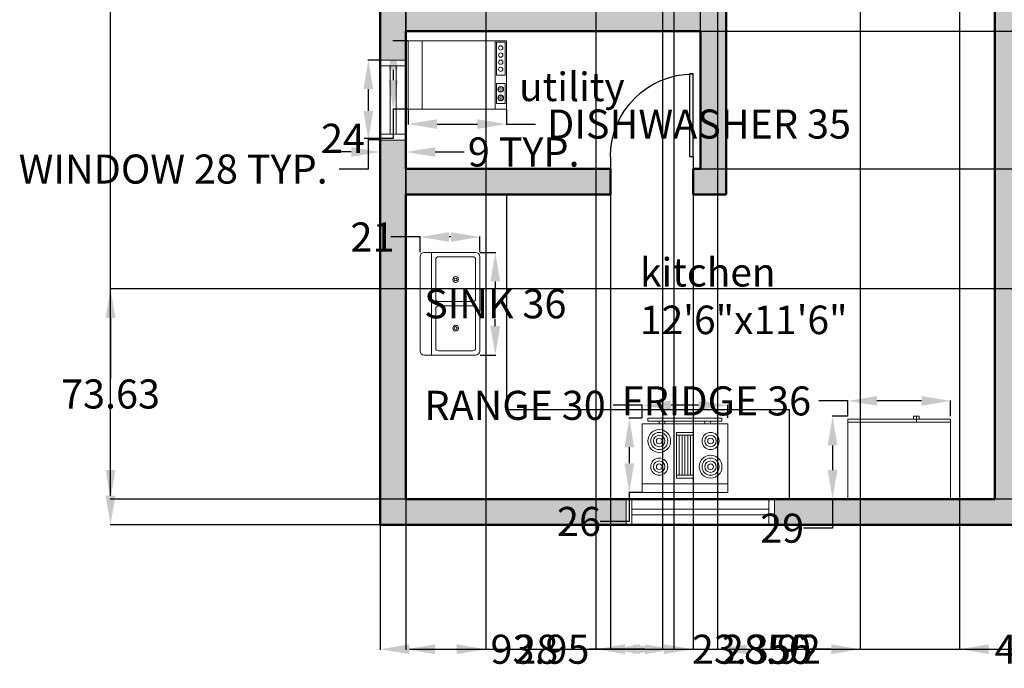
# Model space of a CAD drawing. Units: inches. Extents: x 12496 to 13538, y 6171 to 6892.
# Tile 1 of 6: x 12496 to 12841, y 6171 to 6398. Entities that reach past the tile are written whole.
import ezdxf

# ---------------------------------------------------------------- set-up
doc = ezdxf.new("R2010")
doc.units = ezdxf.units.IN
doc.header["$MEASUREMENT"] = 0
for name, color, linetype, lineweight in [('A-ANNO-DIMS', 2, 'Continuous', 18), ('A-AREA-IDEN', 7, 'Continuous', 25), ('A-DOOR', 3, 'Continuous', 25), ('A-EQPM', 8, 'Continuous', 18), ('A-FLOR-CASE', 8, 'Continuous', 25), ('A-FLOR-FIXT', 9, 'Continuous', 18), ('A-GLAZ', 4, 'Continuous', 18), ('A-WALL', 7, 'Continuous', 50)]:
    doc.layers.add(name, color=color, linetype=linetype, lineweight=lineweight)
doc.layers.add('A-WALL-PATT', color=18, linetype='Continuous', lineweight=13, true_color=0x000000)
doc.styles.get("Standard").update_dxf_attribs({"font": 'arial.ttf'})
doc.dimstyles.get("Standard").update_dxf_attribs({"dimtxt": 10.18, "dimasz": 10.18, "dimexe": 0.18, "dimexo": 0.0625, "dimgap": 0.09, "dimtad": 0, "dimtih": 1, "dimtoh": 1, "dimdec": 0, "dimzin": 0, "dimdsep": 46, "dimlunit": 3, "dimtxsty": 'Standard', "dimcen": 0.09, "dimadec": 0, "dimazin": 0, "dimtfac": 1, "dimtdec": 0, "dimtofl": 0, "dimtmove": 0, "dimatfit": 3, "dimfxl": 1, "dimtolj": 1, "dimtzin": 0, "dimarcsym": 0})

# ---------------------------------------------------------------- blocks, each defined once
blk = doc.blocks.new('Range-Oven - 30 in top')
for p, q in [((0, -3), (30, -3)), ((12, -6), (18, -6)), ((13, -20), (13, -6)), ((14, -6), (14, -20)), ((15, -20), (15, -6)), ((16, -6), (16, -20)), ((17, -20), (17, -6)), ((18, -20), (12, -20)), ((6, -24), (6, -25)), ((8, -25), (8, -24)), ((22, -25), (22, -24)), ((24, -24), (24, -25))]:
    blk.add_line(p, q)
for points in [[(0, -24), (0, 0), (30, 0), (30, -24)], [(12, -21), (12, -5), (18, -5), (18, -21)], [(2, -26), (2, -25), (28, -25), (28, -26)]]:
    blk.add_lwpolyline(points, close=True)
for centre, radius in [((6, -9), 4), ((6, -9), 3), ((24, -9), 3), ((6, -9), 2), ((6, -9), 1), ((24, -9), 2), ((24, -9), 1), ((6, -18), 3), ((6, -18), 2), ((6, -18), 1), ((24, -18), 4), ((24, -18), 3), ((24, -18), 2), ((24, -18), 1)]:
    blk.add_circle(centre, radius)
blk = doc.blocks.new('Sink-double - 36 in top')
for p, q in [((-18, -4), (18, -4)), ((-0.75, -18.5), (-0.75, -6.5)), ((0.75, -6.5), (0.75, -18.5))]:
    blk.add_line(p, q)
for points in [[(-16.5, 0), (16.5, 0)], [(-18, -19.5), (-18, -1.5)], [(18, -1.5), (18, -19.5)], [(-16.5, -18.5), (-16.5, -6.5)], [(-15.5, -5.5), (-1.75, -5.5)], [(1.75, -5.5), (15.5, -5.5)], [(16.5, -6.5), (16.5, -18.5)], [(-1.75, -19.5), (-15.5, -19.5)], [(15.5, -19.5), (1.75, -19.5)], [(16.5, -21), (-16.5, -21)]]:
    blk.add_lwpolyline(points)
for centre, radius in [((-8.5, -12.5), 1), ((-8.5, -12.5), 0.5), ((8.5, -12.5), 1), ((8.5, -12.5), 0.5)]:
    blk.add_circle(centre, radius)
for centre, radius, start, end in [((-16.5, -1.5), 1.5, 90, 180), ((16.5, -1.5), 1.5, 0, 90), ((-15.5, -6.5), 1, 90, 180), ((-1.75, -6.5), 1, 0, 90), ((1.75, -6.5), 1, 90, 180), ((15.5, -6.5), 1, 0, 90), ((-16.5, -19.5), 1.5, 180, 270), ((-15.5, -18.5), 1, 180, 270), ((-1.75, -18.5), 1, 270, 0), ((1.75, -18.5), 1, 180, 270), ((15.5, -18.5), 1, 270, 0), ((16.5, -19.5), 1.5, 270, 0)]:
    blk.add_arc(centre, radius, start, end)
blk = doc.blocks.new('Refrigerator-2 door - 36 in top')
for p, q in [((0, -26.999999), (36, -26.999999)), ((12, -26.999999), (12, -28.999999)), ((11, -27.999999), (11, -28.999999)), ((11, -28.999999), (13, -28.999999)), ((13, -28.999999), (13, -27.999999))]:
    blk.add_line(p, q)
blk.add_lwpolyline([(0, -27.999999), (0, 0), (36, 0), (36, -27.999999)], close=True)
blk = doc.blocks.new('Dishwasher')
for p, q in [((16, 32.5), (16.75, 32.5)), ((16.5, 32), (16.2942, 31.7942)), ((16.3156, 33.1843), (16.5, 33)), ((17, 32.75), (17, 33.5)), ((17, 32.25), (17, 31.5)), ((18, 32.5), (17.25, 32.5)), ((17.5, 33), (17.6938, 33.1938)), ((17.7061, 31.7939), (17.5, 32)), ((19, 32.5), (19.75, 32.5)), ((19.5, 32), (19.2942, 31.7942)), ((19.3156, 33.1843), (19.5, 33)), ((20, 32.75), (20, 33.5)), ((20, 32.25), (20, 31.5)), ((21, 32.5), (20.25, 32.5)), ((20.5, 33), (20.6938, 33.1938)), ((20.7061, 31.7939), (20.5, 32)), ((24, 30.5), (0, 30.5)), ((0, 5), (24, 5))]:
    blk.add_line(p, q)
for points in [[(0, 0), (0, 34.5), (24, 34.5), (24, 0)], [(0.5, 31), (0.5, 34), (12, 34), (12, 31)], [(15, 31), (15, 34), (22, 34), (22, 31)]]:
    blk.add_lwpolyline(points, close=True)
for centre, radius in [((2.5, 32.5), 0.75), ((5, 32.5), 0.75), ((7.5, 32.5), 0.75), ((10, 32.5), 0.75), ((17, 32.5), 1), ((20, 32.5), 1)]:
    blk.add_circle(centre, radius)
blk = doc.blocks.new('*U20')
for p, q in [((0, 0), (0, -6)), ((40, 0), (40, -6))]:
    blk.add_line(p, q)
blk.add_lwpolyline([(0, 0), (0, 40), (1.75, 40), (1.75, 0)], close=True)
blk.add_arc((0, 0), 40, 360, 90)
blk = doc.blocks.new('WIN-48IN')
for p, q in [((0, 0), (0, 9)), ((2, 0), (2, 9)), ((50, 0), (50, 9)), ((52, 0), (52, 9)), ((2, 5.5), (50, 5.5)), ((2, 3.5), (50, 3.5))]:
    blk.add_line(p, q)
blk = doc.blocks.new('WIN-24IN')
for p, q in [((0, 0), (0, 9)), ((2, 0), (2, 9)), ((26, 0), (26, 9)), ((28, 0), (28, 9)), ((2, 5.5), (26, 5.5)), ((2, 3.5), (26, 3.5))]:
    blk.add_line(p, q)
blk = doc.blocks.new('*D33')
at = {"layer": 'A-ANNO-DIMS', "color": 0, "lineweight": -2, "transparency": 16777216}
for p, q in [((12622.11, 6383.69), (12617.79, 6383.69)), ((12617.97, 6373.51), (12617.97, 6365.87)), ((12622.11, 6355.69), (12617.79, 6355.69)), ((12617.97, 6355.69), (12617.97, 6345.51)), ((12617.97, 6345.51), (12607.79, 6345.51))]:
    blk.add_line(p, q, dxfattribs=at)
at = {"layer": 'A-ANNO-DIMS', "color": 0, "transparency": 16777216}
for points in [[(12616.28, 6373.51), (12619.67, 6373.51), (12617.97, 6383.69)], [(12616.28, 6365.87), (12619.67, 6365.87), (12617.97, 6355.69)]]:
    blk.add_solid(points, dxfattribs=at)
at = {"layer": 'Defpoints', "color": 0, "transparency": 16777216}
for p in [(12622.17, 6383.69), (12617.97, 6355.69), (12622.17, 6355.69)]:
    blk.add_point(p, dxfattribs=at)
at = {"layer": 'A-ANNO-DIMS', "color": 0, "transparency": 16777216, "insert": (12549.54, 6345.51), "char_height": 10.18, "attachment_point": 5}
blk.add_mtext('\\A1;WINDOW 28 TYP.', dxfattribs=at)
blk = doc.blocks.new('*D34')
at = {"layer": 'A-ANNO-DIMS', "color": 0, "lineweight": -2, "transparency": 16777216}
for p, q in [((12622.17, 6355.62), (12622.17, 6351.31)), ((12631.17, 6355.62), (12631.17, 6351.31)), ((12611.99, 6351.49), (12601.81, 6351.49)), ((12641.35, 6351.49), (12651.53, 6351.49))]:
    blk.add_line(p, q, dxfattribs=at)
at = {"layer": 'A-ANNO-DIMS', "color": 0, "transparency": 16777216}
for points in [[(12611.99, 6353.18), (12611.99, 6349.79), (12622.17, 6351.49)], [(12641.35, 6353.18), (12641.35, 6349.79), (12631.17, 6351.49)]]:
    blk.add_solid(points, dxfattribs=at)
at = {"layer": 'Defpoints', "color": 0, "transparency": 16777216}
for p in [(12622.17, 6355.69), (12631.17, 6355.69), (12631.17, 6351.49)]:
    blk.add_point(p, dxfattribs=at)
at = {"layer": 'A-ANNO-DIMS', "color": 0, "transparency": 16777216, "insert": (12672.44, 6351.49), "char_height": 10.18, "attachment_point": 5}
blk.add_mtext('\\A1;9 TYP.', dxfattribs=at)
blk = doc.blocks.new('*D45')
at = {"layer": 'A-ANNO-DIMS', "color": 0, "lineweight": -2, "transparency": 16777216}
for p, q in [((12713.97, 6262.74), (12703.79, 6262.74)), ((12713.97, 6258.31), (12713.97, 6262.92)), ((12733.79, 6262.74), (12724.15, 6262.74)), ((12743.97, 6258.31), (12743.97, 6262.92))]:
    blk.add_line(p, q, dxfattribs=at)
at = {"layer": 'A-ANNO-DIMS', "color": 0, "transparency": 16777216}
for points in [[(12724.15, 6264.44), (12724.15, 6261.05), (12713.97, 6262.74)], [(12733.79, 6264.44), (12733.79, 6261.05), (12743.97, 6262.74)]]:
    blk.add_solid(points, dxfattribs=at)
at = {"layer": 'Defpoints', "color": 0, "transparency": 16777216}
for p in [(12713.97, 6262.74), (12713.97, 6258.24), (12743.97, 6258.24)]:
    blk.add_point(p, dxfattribs=at)
at = {"layer": 'A-ANNO-DIMS', "color": 0, "transparency": 16777216, "insert": (12669.43, 6262.74), "char_height": 10.18, "attachment_point": 5}
blk.add_mtext('\\A1;RANGE 30', dxfattribs=at)
blk = doc.blocks.new('*D46')
at = {"layer": 'A-ANNO-DIMS', "color": 0, "lineweight": -2, "transparency": 16777216}
for p, q in [((12713.91, 6258.24), (12709.29, 6258.24)), ((12709.47, 6248.06), (12709.47, 6242.42)), ((12713.91, 6232.24), (12709.29, 6232.24)), ((12709.47, 6232.24), (12709.47, 6222.06)), ((12709.47, 6222.06), (12699.29, 6222.06))]:
    blk.add_line(p, q, dxfattribs=at)
at = {"layer": 'A-ANNO-DIMS', "color": 0, "transparency": 16777216}
for points in [[(12707.77, 6248.06), (12711.17, 6248.06), (12709.47, 6258.24)], [(12707.77, 6242.42), (12711.17, 6242.42), (12709.47, 6232.24)]]:
    blk.add_solid(points, dxfattribs=at)
at = {"layer": 'Defpoints', "color": 0, "transparency": 16777216}
for p in [(12713.97, 6258.24), (12709.47, 6232.24), (12713.97, 6232.24)]:
    blk.add_point(p, dxfattribs=at)
at = {"layer": 'A-ANNO-DIMS', "color": 0, "transparency": 16777216, "insert": (12691.83, 6222.06), "char_height": 10.18, "attachment_point": 5}
blk.add_mtext('\\A1;26', dxfattribs=at)
blk = doc.blocks.new('*D47')
at = {"layer": 'A-ANNO-DIMS', "color": 0, "lineweight": -2, "transparency": 16777216}
for p, q in [((12657.15, 6316.31), (12662.67, 6316.31)), ((12662.49, 6306.13), (12662.49, 6303.67)), ((12662.49, 6290.49), (12662.49, 6292.96)), ((12657.15, 6280.31), (12662.67, 6280.31))]:
    blk.add_line(p, q, dxfattribs=at)
at = {"layer": 'A-ANNO-DIMS', "color": 0, "transparency": 16777216}
for points in [[(12660.79, 6306.13), (12664.19, 6306.13), (12662.49, 6316.31)], [(12660.79, 6290.49), (12664.19, 6290.49), (12662.49, 6280.31)]]:
    blk.add_solid(points, dxfattribs=at)
at = {"layer": 'Defpoints', "color": 0, "transparency": 16777216}
for p in [(12657.09, 6316.31), (12662.49, 6316.31), (12657.09, 6280.31)]:
    blk.add_point(p, dxfattribs=at)
at = {"layer": 'A-ANNO-DIMS', "color": 0, "transparency": 16777216, "insert": (12662.49, 6298.31), "char_height": 10.18, "attachment_point": 5}
blk.add_mtext('\\A1;SINK 36', dxfattribs=at)
blk = doc.blocks.new('*D48')
at = {"layer": 'A-ANNO-DIMS', "color": 0, "lineweight": -2, "transparency": 16777216}
for p, q in [((12636.09, 6321.71), (12625.91, 6321.71)), ((12636.09, 6316.38), (12636.09, 6321.89)), ((12646.91, 6321.71), (12646.27, 6321.71)), ((12657.09, 6316.38), (12657.09, 6321.89))]:
    blk.add_line(p, q, dxfattribs=at)
at = {"layer": 'A-ANNO-DIMS', "color": 0, "transparency": 16777216}
for points in [[(12646.27, 6323.41), (12646.27, 6320.02), (12636.09, 6321.71)], [(12646.91, 6323.41), (12646.91, 6320.02), (12657.09, 6321.71)]]:
    blk.add_solid(points, dxfattribs=at)
at = {"layer": 'Defpoints', "color": 0, "transparency": 16777216}
for p in [(12636.09, 6321.71), (12636.09, 6316.31), (12657.09, 6316.31)]:
    blk.add_point(p, dxfattribs=at)
at = {"layer": 'A-ANNO-DIMS', "color": 0, "transparency": 16777216, "insert": (12619.42, 6321.71), "char_height": 10.18, "attachment_point": 5}
blk.add_mtext('\\A1;21', dxfattribs=at)
blk = doc.blocks.new('*D49')
at = {"layer": 'A-ANNO-DIMS', "color": 0, "lineweight": -2, "transparency": 16777216}
for p, q in [((12786.13, 6264.29), (12775.95, 6264.29)), ((12786.13, 6258.96), (12786.13, 6264.47)), ((12811.95, 6264.29), (12796.31, 6264.29)), ((12822.13, 6258.96), (12822.13, 6264.47))]:
    blk.add_line(p, q, dxfattribs=at)
at = {"layer": 'A-ANNO-DIMS', "color": 0, "transparency": 16777216}
for points in [[(12796.31, 6265.99), (12796.31, 6262.6), (12786.13, 6264.29)], [(12811.95, 6265.99), (12811.95, 6262.6), (12822.13, 6264.29)]]:
    blk.add_solid(points, dxfattribs=at)
at = {"layer": 'Defpoints', "color": 0, "transparency": 16777216}
for p in [(12786.13, 6264.29), (12786.13, 6258.89), (12822.13, 6258.89)]:
    blk.add_point(p, dxfattribs=at)
at = {"layer": 'A-ANNO-DIMS', "color": 0, "transparency": 16777216, "insert": (12740.02, 6264.29), "char_height": 10.18, "attachment_point": 5}
blk.add_mtext('\\A1;FRIDGE 36', dxfattribs=at)
blk = doc.blocks.new('*D50')
at = {"layer": 'A-ANNO-DIMS', "color": 0, "lineweight": -2, "transparency": 16777216}
for p, q in [((12786.07, 6258.89), (12780.55, 6258.89)), ((12780.73, 6248.71), (12780.73, 6240.07)), ((12786.07, 6229.89), (12780.55, 6229.89)), ((12780.73, 6229.89), (12780.73, 6219.71)), ((12780.73, 6219.71), (12770.55, 6219.71))]:
    blk.add_line(p, q, dxfattribs=at)
at = {"layer": 'A-ANNO-DIMS', "color": 0, "transparency": 16777216}
for points in [[(12779.03, 6248.71), (12782.43, 6248.71), (12780.73, 6258.89)], [(12779.03, 6240.07), (12782.43, 6240.07), (12780.73, 6229.89)]]:
    blk.add_solid(points, dxfattribs=at)
at = {"layer": 'Defpoints', "color": 0, "transparency": 16777216}
for p in [(12786.13, 6258.89), (12780.73, 6229.89), (12786.13, 6229.89)]:
    blk.add_point(p, dxfattribs=at)
at = {"layer": 'A-ANNO-DIMS', "color": 0, "transparency": 16777216, "insert": (12763.07, 6219.71), "char_height": 10.18, "attachment_point": 5}
blk.add_mtext('\\A1;29', dxfattribs=at)
blk = doc.blocks.new('*D57')
at = {"layer": 'A-ANNO-DIMS', "color": 0, "lineweight": -2, "transparency": 16777216}
for p, q in [((12631.9, 6366.38), (12631.9, 6361.09)), ((12666.4, 6366.38), (12666.4, 6361.09)), ((12642.08, 6361.27), (12656.22, 6361.27)), ((12666.4, 6361.27), (12676.58, 6361.27))]:
    blk.add_line(p, q, dxfattribs=at)
at = {"layer": 'A-ANNO-DIMS', "color": 0, "transparency": 16777216}
for points in [[(12642.08, 6362.97), (12642.08, 6359.57), (12631.9, 6361.27)], [(12656.22, 6362.97), (12656.22, 6359.57), (12666.4, 6361.27)]]:
    blk.add_solid(points, dxfattribs=at)
at = {"layer": 'Defpoints', "color": 0, "transparency": 16777216}
for p in [(12631.9, 6366.45), (12666.4, 6366.45), (12666.4, 6361.27)]:
    blk.add_point(p, dxfattribs=at)
at = {"layer": 'A-ANNO-DIMS', "color": 0, "transparency": 16777216, "insert": (12733.92, 6361.27), "char_height": 10.18, "attachment_point": 5}
blk.add_mtext('\\A1;DISHWASHER 35', dxfattribs=at)
blk = doc.blocks.new('*D58')
at = {"layer": 'A-ANNO-DIMS', "color": 0, "lineweight": -2, "transparency": 16777216}
for p, q in [((12631.84, 6390.45), (12626.55, 6390.45)), ((12626.73, 6380.27), (12626.73, 6376.63)), ((12631.84, 6366.45), (12626.55, 6366.45)), ((12626.73, 6366.45), (12626.73, 6356.27)), ((12626.73, 6356.27), (12616.55, 6356.27))]:
    blk.add_line(p, q, dxfattribs=at)
at = {"layer": 'A-ANNO-DIMS', "color": 0, "transparency": 16777216}
for points in [[(12625.03, 6380.27), (12628.42, 6380.27), (12626.73, 6390.45)], [(12625.03, 6376.63), (12628.42, 6376.63), (12626.73, 6366.45)]]:
    blk.add_solid(points, dxfattribs=at)
at = {"layer": 'Defpoints', "color": 0, "transparency": 16777216}
for p in [(12631.9, 6390.45), (12626.73, 6366.45), (12631.9, 6366.45)]:
    blk.add_point(p, dxfattribs=at)
at = {"layer": 'A-ANNO-DIMS', "color": 0, "transparency": 16777216, "insert": (12609.1, 6356.27), "char_height": 10.18, "attachment_point": 5}
blk.add_mtext('\\A1;24', dxfattribs=at)
blk = doc.blocks.new('*D59')
at = {"layer": 'A-ANNO-DIMS', "color": 0, "lineweight": -2, "transparency": 16777216}
for p, q in [((12622.17, 6220.83), (12622.17, 6177.12)), ((13443.03, 6220.83), (13443.03, 6177.12)), ((12632.35, 6177.3), (13015.32, 6177.3)), ((13432.85, 6177.3), (13049.88, 6177.3))]:
    blk.add_line(p, q, dxfattribs=at)
at = {"layer": 'A-ANNO-DIMS', "color": 0, "transparency": 16777216}
for points in [[(12632.35, 6179), (12632.35, 6175.6), (12622.17, 6177.3)], [(13432.85, 6179), (13432.85, 6175.6), (13443.03, 6177.3)]]:
    blk.add_solid(points, dxfattribs=at)
at = {"layer": 'Defpoints', "color": 0, "transparency": 16777216}
for p in [(12622.17, 6220.89), (13443.03, 6220.89), (13443.03, 6177.3)]:
    blk.add_point(p, dxfattribs=at)
at = {"layer": 'A-ANNO-DIMS', "color": 0, "transparency": 16777216, "insert": (13032.6, 6177.3), "char_height": 10.18, "attachment_point": 5}
blk.add_mtext('\\A1;820.9', dxfattribs=at)
blk = doc.blocks.new('*D60')
at = {"layer": 'A-ANNO-DIMS', "color": 0, "lineweight": -2, "transparency": 16777216}
for p, q in [((12622.11, 6790.89), (12527.4, 6790.89)), ((12527.58, 6780.71), (12527.58, 6511.18)), ((12527.58, 6231.07), (12527.58, 6500.61)), ((12622.11, 6220.89), (12527.4, 6220.89))]:
    blk.add_line(p, q, dxfattribs=at)
at = {"layer": 'A-ANNO-DIMS', "color": 0, "transparency": 16777216}
for points in [[(12525.88, 6780.71), (12529.28, 6780.71), (12527.58, 6790.89)], [(12525.88, 6231.07), (12529.28, 6231.07), (12527.58, 6220.89)]]:
    blk.add_solid(points, dxfattribs=at)
at = {"layer": 'Defpoints', "color": 0, "transparency": 16777216}
for p in [(12527.58, 6790.89), (12622.17, 6790.89), (12622.17, 6220.89)]:
    blk.add_point(p, dxfattribs=at)
at = {"layer": 'A-ANNO-DIMS', "color": 0, "transparency": 16777216, "insert": (12527.58, 6505.89), "char_height": 10.18, "attachment_point": 5}
blk.add_mtext('\\A1;570', dxfattribs=at)
blk = doc.blocks.new('*D65')
at = {"layer": 'A-ANNO-DIMS', "color": 0, "lineweight": -2, "transparency": 16777216}
for p, q in [((12631.17, 6229.96), (12631.17, 6885.67)), ((12641.35, 6885.49), (12713.08, 6885.49)), ((12827.42, 6885.49), (12755.7, 6885.49)), ((12837.6, 6229.96), (12837.6, 6885.67))]:
    blk.add_line(p, q, dxfattribs=at)
at = {"layer": 'A-ANNO-DIMS', "color": 0, "transparency": 16777216}
for points in [[(12641.35, 6887.18), (12641.35, 6883.79), (12631.17, 6885.49)], [(12827.42, 6887.18), (12827.42, 6883.79), (12837.6, 6885.49)]]:
    blk.add_solid(points, dxfattribs=at)
at = {"layer": 'Defpoints', "color": 0, "transparency": 16777216}
for p in [(12837.6, 6885.49), (12631.17, 6229.89), (12837.6, 6229.89)]:
    blk.add_point(p, dxfattribs=at)
at = {"layer": 'A-ANNO-DIMS', "color": 0, "transparency": 16777216, "insert": (12734.39, 6885.49), "char_height": 10.18, "attachment_point": 5}
blk.add_mtext('\\A1;206.43', dxfattribs=at)
blk = doc.blocks.new('*D71')
at = {"layer": 'A-ANNO-DIMS', "color": 0, "lineweight": -2, "transparency": 16777216}
for p, q in [((13109.04, 6303.52), (12527.4, 6303.52)), ((12527.58, 6293.34), (12527.58, 6272)), ((12527.58, 6240.07), (12527.58, 6261.42)), ((13109.04, 6229.89), (12527.4, 6229.89))]:
    blk.add_line(p, q, dxfattribs=at)
at = {"layer": 'A-ANNO-DIMS', "color": 0, "transparency": 16777216}
for points in [[(12525.88, 6293.34), (12529.28, 6293.34), (12527.58, 6303.52)], [(12525.88, 6240.07), (12529.28, 6240.07), (12527.58, 6229.89)]]:
    blk.add_solid(points, dxfattribs=at)
at = {"layer": 'Defpoints', "color": 0, "transparency": 16777216}
for p in [(12527.58, 6303.52), (13109.1, 6303.52), (13109.1, 6229.89)]:
    blk.add_point(p, dxfattribs=at)
at = {"layer": 'A-ANNO-DIMS', "color": 0, "transparency": 16777216, "insert": (12527.58, 6266.71), "char_height": 10.18, "attachment_point": 5}
blk.add_mtext('\\A1;73.63', dxfattribs=at)
blk = doc.blocks.new('*D72')
at = {"layer": 'A-ANNO-DIMS', "color": 0, "lineweight": -2, "transparency": 16777216}
for p, q in [((12734.45, 6393.81), (13486.8, 6393.81)), ((13486.62, 6383.63), (13486.62, 6374.97)), ((13486.62, 6355.74), (13486.62, 6364.4)), ((12734.45, 6345.56), (13486.8, 6345.56))]:
    blk.add_line(p, q, dxfattribs=at)
at = {"layer": 'A-ANNO-DIMS', "color": 0, "transparency": 16777216}
for points in [[(13484.92, 6383.63), (13488.32, 6383.63), (13486.62, 6393.81)], [(13484.92, 6355.74), (13488.32, 6355.74), (13486.62, 6345.56)]]:
    blk.add_solid(points, dxfattribs=at)
at = {"layer": 'Defpoints', "color": 0, "transparency": 16777216}
for p in [(12734.39, 6393.81), (13486.62, 6393.81), (12734.39, 6345.56)]:
    blk.add_point(p, dxfattribs=at)
at = {"layer": 'A-ANNO-DIMS', "color": 0, "transparency": 16777216, "insert": (13486.62, 6369.69), "char_height": 10.18, "attachment_point": 5}
blk.add_mtext('\\A1;48.25', dxfattribs=at)
blk = doc.blocks.new('*D73')
at = {"layer": 'A-ANNO-DIMS', "color": 0, "lineweight": -2, "transparency": 16777216}
for p, q in [((12631.17, 6393.87), (12631.17, 6885.67)), ((12641.35, 6885.49), (12663.02, 6885.49)), ((12724.21, 6885.49), (12702.54, 6885.49)), ((12734.39, 6393.87), (12734.39, 6885.67))]:
    blk.add_line(p, q, dxfattribs=at)
at = {"layer": 'A-ANNO-DIMS', "color": 0, "transparency": 16777216}
for points in [[(12641.35, 6887.18), (12641.35, 6883.79), (12631.17, 6885.49)], [(12724.21, 6887.18), (12724.21, 6883.79), (12734.39, 6885.49)]]:
    blk.add_solid(points, dxfattribs=at)
at = {"layer": 'Defpoints', "color": 0, "transparency": 16777216}
for p in [(12734.39, 6885.49), (12631.17, 6393.81), (12734.39, 6393.81)]:
    blk.add_point(p, dxfattribs=at)
at = {"layer": 'A-ANNO-DIMS', "color": 0, "transparency": 16777216, "insert": (12682.78, 6885.49), "char_height": 10.18, "attachment_point": 5}
blk.add_mtext('\\A1;103.21', dxfattribs=at)
blk = doc.blocks.new('*D74')
at = {"layer": 'A-ANNO-DIMS', "color": 0, "lineweight": -2, "transparency": 16777216}
for p, q in [((12702.9, 6345.5), (12702.9, 6177.12)), ((12731.82, 6345.5), (12731.82, 6177.12)), ((12713.08, 6177.3), (12721.64, 6177.3)), ((12731.82, 6177.3), (12742, 6177.3))]:
    blk.add_line(p, q, dxfattribs=at)
at = {"layer": 'A-ANNO-DIMS', "color": 0, "transparency": 16777216}
for points in [[(12713.08, 6179), (12713.08, 6175.6), (12702.9, 6177.3)], [(12721.64, 6179), (12721.64, 6175.6), (12731.82, 6177.3)]]:
    blk.add_solid(points, dxfattribs=at)
at = {"layer": 'Defpoints', "color": 0, "transparency": 16777216}
for p in [(12702.9, 6345.56), (12731.82, 6345.56), (12731.82, 6177.3)]:
    blk.add_point(p, dxfattribs=at)
at = {"layer": 'A-ANNO-DIMS', "color": 0, "transparency": 16777216, "insert": (12759.3, 6177.3), "char_height": 10.18, "attachment_point": 5}
blk.add_mtext('\\A1;28.92', dxfattribs=at)
blk = doc.blocks.new('*D77')
at = {"layer": 'A-ANNO-DIMS', "color": 0, "lineweight": -2, "transparency": 16777216}
for p, q in [((12697.73, 6559.71), (12697.73, 6177.12)), ((12721.09, 6560.6), (12721.09, 6177.12)), ((12707.91, 6177.3), (12710.91, 6177.3)), ((12721.09, 6177.3), (12731.27, 6177.3))]:
    blk.add_line(p, q, dxfattribs=at)
at = {"layer": 'A-ANNO-DIMS', "color": 0, "transparency": 16777216}
for points in [[(12707.91, 6179), (12707.91, 6175.6), (12697.73, 6177.3)], [(12710.91, 6179), (12710.91, 6175.6), (12721.09, 6177.3)]]:
    blk.add_solid(points, dxfattribs=at)
at = {"layer": 'Defpoints', "color": 0, "transparency": 16777216}
for p in [(12697.73, 6559.77), (12721.09, 6560.66), (12721.09, 6177.3)]:
    blk.add_point(p, dxfattribs=at)
at = {"layer": 'A-ANNO-DIMS', "color": 0, "transparency": 16777216, "insert": (12752.61, 6177.3), "char_height": 10.18, "attachment_point": 5}
blk.add_mtext('\\A1;23.355', dxfattribs=at)
blk = doc.blocks.new('*D79')
at = {"layer": 'A-ANNO-DIMS', "color": 0, "lineweight": -2, "transparency": 16777216}
for p, q in [((12659.17, 6539.09), (12659.17, 6177.12)), ((12631.17, 6528.59), (12631.17, 6177.12)), ((12641.35, 6177.3), (12648.99, 6177.3)), ((12659.17, 6177.3), (12669.35, 6177.3))]:
    blk.add_line(p, q, dxfattribs=at)
at = {"layer": 'A-ANNO-DIMS', "color": 0, "transparency": 16777216}
for points in [[(12641.35, 6179), (12641.35, 6175.6), (12631.17, 6177.3)], [(12648.99, 6179), (12648.99, 6175.6), (12659.17, 6177.3)]]:
    blk.add_solid(points, dxfattribs=at)
at = {"layer": 'Defpoints', "color": 0, "transparency": 16777216}
for p in [(12659.17, 6539.15), (12631.17, 6528.65), (12659.17, 6177.3)]:
    blk.add_point(p, dxfattribs=at)
at = {"layer": 'A-ANNO-DIMS', "color": 0, "transparency": 16777216, "insert": (12676.83, 6177.3), "char_height": 10.18, "attachment_point": 5}
blk.add_mtext('\\A1;28', dxfattribs=at)
blk = doc.blocks.new('*D80')
at = {"layer": 'A-ANNO-DIMS', "color": 0, "lineweight": -2, "transparency": 16777216}
for p, q in [((12631.17, 6781.83), (12631.17, 6177.12)), ((12725.12, 6781.83), (12725.12, 6177.12)), ((12641.35, 6177.3), (12660.84, 6177.3)), ((12714.94, 6177.3), (12695.45, 6177.3))]:
    blk.add_line(p, q, dxfattribs=at)
at = {"layer": 'A-ANNO-DIMS', "color": 0, "transparency": 16777216}
for points in [[(12641.35, 6179), (12641.35, 6175.6), (12631.17, 6177.3)], [(12714.94, 6179), (12714.94, 6175.6), (12725.12, 6177.3)]]:
    blk.add_solid(points, dxfattribs=at)
at = {"layer": 'Defpoints', "color": 0, "transparency": 16777216}
for p in [(12631.17, 6781.89), (12725.12, 6781.89), (12725.12, 6177.3)]:
    blk.add_point(p, dxfattribs=at)
at = {"layer": 'A-ANNO-DIMS', "color": 0, "transparency": 16777216, "insert": (12678.15, 6177.3), "char_height": 10.18, "attachment_point": 5}
blk.add_mtext('\\A1;93.95', dxfattribs=at)
blk = doc.blocks.new('*D86')
at = {"layer": 'A-ANNO-DIMS', "color": 0, "lineweight": -2, "transparency": 16777216}
for p, q in [((12740.45, 6507.47), (12740.45, 6177.12)), ((12790.45, 6507.47), (12790.45, 6177.12)), ((12750.63, 6177.3), (12758.09, 6177.3)), ((12780.27, 6177.3), (12772.81, 6177.3))]:
    blk.add_line(p, q, dxfattribs=at)
at = {"layer": 'A-ANNO-DIMS', "color": 0, "transparency": 16777216}
for points in [[(12750.63, 6179), (12750.63, 6175.6), (12740.45, 6177.3)], [(12780.27, 6179), (12780.27, 6175.6), (12790.45, 6177.3)]]:
    blk.add_solid(points, dxfattribs=at)
at = {"layer": 'Defpoints', "color": 0, "transparency": 16777216}
for p in [(12740.45, 6507.54), (12790.45, 6507.54), (12790.45, 6177.3)]:
    blk.add_point(p, dxfattribs=at)
at = {"layer": 'A-ANNO-DIMS', "color": 0, "transparency": 16777216, "insert": (12765.45, 6177.3), "char_height": 10.18, "attachment_point": 5}
blk.add_mtext('\\A1;50', dxfattribs=at)
blk = doc.blocks.new('*D87')
at = {"layer": 'A-ANNO-DIMS', "color": 0, "lineweight": -2, "transparency": 16777216}
for p, q in [((12825.27, 6572.14), (12825.27, 6177.12)), ((12865.27, 6572.14), (12865.27, 6177.12)), ((12835.45, 6177.3), (12837.7, 6177.3)), ((12855.09, 6177.3), (12852.83, 6177.3))]:
    blk.add_line(p, q, dxfattribs=at)
at = {"layer": 'A-ANNO-DIMS', "color": 0, "transparency": 16777216}
for points in [[(12835.45, 6179), (12835.45, 6175.6), (12825.27, 6177.3)], [(12855.09, 6179), (12855.09, 6175.6), (12865.27, 6177.3)]]:
    blk.add_solid(points, dxfattribs=at)
at = {"layer": 'Defpoints', "color": 0, "transparency": 16777216}
for p in [(12825.27, 6572.2), (12865.27, 6572.2), (12865.27, 6177.3)]:
    blk.add_point(p, dxfattribs=at)
at = {"layer": 'A-ANNO-DIMS', "color": 0, "transparency": 16777216, "insert": (12845.27, 6177.3), "char_height": 10.18, "attachment_point": 5}
blk.add_mtext('\\A1;40', dxfattribs=at)

msp = doc.modelspace()

# ---------------------------------------------------------------- hatches: boundary and pattern name
at = {"layer": 'A-WALL-PATT'}
h = msp.add_hatch(color=256, dxfattribs=at)
h.dxf.hatch_style = 1
h.paths.add_polyline_path([(13443.0285, 6790.8943), (13327.7025, 6790.8943), (13327.7025, 6781.8943), (13434.0285, 6781.8943), (13434.0285, 6572.2028), (13169.3765, 6572.2028), (13169.3765, 6576.9323), (13160.3765, 6576.9323), (13160.3765, 6563.2028), (13163.811, 6563.2028), (13163.811, 6559.305), (13172.811, 6559.305), (13172.811, 6563.2028), (13434.0285, 6563.2028), (13434.0285, 6402.794), (13331.4198, 6402.794), (13331.4198, 6393.8103), (13434.0285, 6393.8103), (13434.0285, 6220.8943), (13443.0285, 6220.8943)])
h.paths.add_polyline_path([(13172.811, 6519.305), (13163.811, 6519.305), (13163.811, 6402.8103), (12944.6655, 6402.8103), (12944.6655, 6393.8103), (13100.0985, 6393.8103), (13100.0985, 6312.5223), (13035.7682, 6312.5223), (13035.7682, 6303.5223), (13109.0985, 6303.5223), (13109.0985, 6393.8103), (13279.4198, 6393.8103), (13279.4198, 6402.8103), (13172.811, 6402.8103)])
h.paths.add_polyline_path([(13109.0985, 6229.8943), (12846.603, 6229.8943), (12846.603, 6303.5223), (12853.6371, 6303.5223), (12853.6371, 6312.5223), (12846.603, 6312.5223), (12846.603, 6393.8103), (12872.7237, 6393.8103), (12872.7237, 6402.8103), (12846.603, 6402.8103), (12837.603, 6402.8103), (12837.603, 6229.8943), (12760.3881, 6229.8943), (12760.3881, 6220.8943), (13109.0985, 6220.8943)])
h.paths.add_polyline_path([(12708.3881, 6229.8943), (12631.1731, 6229.8943), (12631.1731, 6336.5598), (12702.8967, 6336.5598), (12702.8967, 6345.5598), (12631.1731, 6345.5598), (12631.1731, 6355.6851), (12622.1731, 6355.6851), (12622.1731, 6220.8943), (12708.3881, 6220.8943)])
h.paths.add_polyline_path([(12743.3881, 6402.8103), (12631.1731, 6402.8103), (12631.1731, 6523.6486), (12622.1731, 6523.6486), (12622.1731, 6383.6851), (12631.1731, 6383.6851), (12631.1731, 6393.8103), (12734.3881, 6393.8103), (12734.3881, 6345.5598), (12731.8151, 6345.5598), (12731.8151, 6336.5598), (12734.3881, 6336.5598), (12743.3881, 6336.5598)])
h.paths.add_polyline_path([(13039.9206, 6572.2028), (13039.9206, 6638.8628), (13048.7069, 6638.8628), (13048.7069, 6647.8628), (13039.9206, 6647.8628), (12930.9211, 6647.8628), (12930.9211, 6638.8628), (13030.9206, 6638.8628), (13030.9206, 6572.2028), (12880.0706, 6572.2028), (12880.0706, 6576.9323), (12871.0706, 6576.9323), (12871.0706, 6572.2028), (12865.2657, 6572.2028), (12865.2657, 6563.2028), (13039.9206, 6563.2028)])
h.paths.add_polyline_path([(13039.9206, 6781.8943), (13086.1485, 6781.8943), (13086.1485, 6790.8943), (12969.4956, 6790.8943), (12969.4956, 6781.8943), (13030.9206, 6781.8943), (13030.9206, 6647.8628), (13039.9206, 6647.8628)])
h.paths.add_polyline_path([(13169.3765, 6781.8943), (13275.7025, 6781.8943), (13275.7025, 6790.8943), (13114.1485, 6790.8943), (13114.1485, 6781.8943), (13160.3765, 6781.8943), (13160.3765, 6647.8628), (13088.7069, 6647.8628), (13088.7069, 6638.8628), (13160.3765, 6638.8628), (13160.3765, 6616.9323), (13169.3765, 6616.9323)])

# ---------------------------------------------------------------- linework, layer by layer
at = {"layer": 'A-FLOR-CASE'}
for p, q in [((12666.3697, 6336.5598), (12666.3697, 6261.3229)), ((12666.3697, 6261.3229), (12765.5234, 6261.3229)), ((12765.5234, 6261.3229), (12765.5234, 6229.8943))]:
    msp.add_line(p, q, dxfattribs=at)
at = {"layer": 'A-WALL'}
for p, q in [((12622.1731, 6220.8943), (12622.1731, 6790.8943)), ((12743.3881, 6402.8103), (12743.3881, 6336.5598)), ((12837.603, 6229.8943), (12837.603, 6402.8103)), ((12631.1731, 6393.8103), (12734.3881, 6393.8103)), ((12631.1731, 6345.5598), (12631.1731, 6393.8103)), ((12734.3881, 6393.8103), (12734.3881, 6345.5598)), ((12631.1731, 6345.5598), (12631.1731, 6345.5598)), ((12631.1731, 6345.5598), (12702.8967, 6345.5598)), ((12702.8967, 6345.5598), (12702.8967, 6336.5598)), ((12731.8151, 6345.5598), (12734.3881, 6345.5598)), ((12731.8151, 6345.5598), (12731.8151, 6336.5598)), ((12631.1731, 6229.8943), (12631.1731, 6336.5598)), ((12631.1731, 6336.5598), (12702.8967, 6336.5598)), ((12731.8151, 6336.5598), (12734.3881, 6336.5598)), ((12734.3881, 6336.5598), (12743.3881, 6336.5598)), ((12631.1731, 6229.8943), (12837.603, 6229.8943)), ((12622.1731, 6220.8943), (13109.0985, 6220.8943))]:
    msp.add_line(p, q, dxfattribs=at)

# ---------------------------------------------------------------- block references
at = {"layer": 'A-DOOR', "xscale": -0.7229599162244675, "yscale": 0.7229599162244675, "zscale": 0.7229599162244675}
msp.add_blockref('*U20', (12731.8151, 6349.8976), dxfattribs=at)
at = {"layer": 'A-EQPM'}
for name, p, rotation in [('Dishwasher', (12631.9027, 6390.4455), 270), ('Refrigerator-2 door - 36 in top', (12822.1307, 6229.8943), 180), ('Range-Oven - 30 in top', (12743.9709, 6232.2446), 180)]:
    msp.add_blockref(name, p, dxfattribs=dict(at, rotation=rotation))
at = {"layer": 'A-FLOR-FIXT', "rotation": 90}
msp.add_blockref('Sink-double - 36 in top', (12636.0891, 6298.3142), dxfattribs=at)
at = {"layer": 'A-GLAZ'}
for name, p, rotation in [('WIN-24IN', (12622.1727, 6383.6847), 269.9999999999955), ('WIN-48IN', (12760.3879, 6229.8947), 180)]:
    msp.add_blockref(name, p, dxfattribs=dict(at, rotation=rotation))

# ---------------------------------------------------------------- texts
at = {"layer": 'A-AREA-IDEN', "char_height": 10, "attachment_point": 1}
for s, insert in [('utility', (12670.8077, 6379.3114)), ('kitchen\\P12\'6"x11\'6"', (12713.2351, 6314.3467))]:
    msp.add_mtext_dynamic_manual_height_columns(s, width=261.947845, gutter_width=1, heights=[0], dxfattribs=dict(at, insert=insert))

# ---------------------------------------------------------------- dimensions: what is measured, and where the dimension line sits
at = {"layer": 'A-ANNO-DIMS'}
for base, p1, p2, override, picture, middle in [((12837.603, 6885.4873), (12631.1731, 6229.8943), (12837.603, 6229.8943), {"dimdec": 2, "dimlfac": 1, "dimrnd": 0, "dimzin": 0, "dimdsep": 46, "dimlunit": 2}, '*D65', (12734.3881, 6885.4873)), ((12734.38807, 6885.48735), (12631.17309, 6393.81032), (12734.38807, 6393.81032), {"dimdec": 2, "dimlfac": 1, "dimrnd": 0, "dimzin": 0, "dimdsep": 46, "dimlunit": 2}, '*D73', (12682.78058, 6885.48735)), ((12725.1219, 6177.3013), (12631.1731, 6781.8943), (12725.1219, 6781.8943), {"dimdec": 2, "dimlfac": 1, "dimrnd": 0, "dimzin": 0, "dimdsep": 46, "dimlunit": 2}, '*D80', (12678.1475, 6177.3013)), ((12865.2657, 6177.3013), (12825.2657, 6572.2028), (12865.2657, 6572.2028), {"dimdec": 0, "dimlfac": 1, "dimrnd": 0, "dimzin": 0, "dimdsep": 46, "dimlunit": 2}, '*D87', (12845.2657, 6177.3013)), ((12721.0852, 6177.3013), (12697.7301, 6559.7717), (12721.0852, 6560.6603), {"dimdec": 3, "dimlfac": 1, "dimrnd": 0, "dimzin": 0, "dimdsep": 46, "dimlunit": 2}, '*D77', (12752.611, 6177.3013)), ((12659.1731, 6177.3013), (12631.1731, 6528.6486), (12659.1731, 6539.1487), {"dimdec": 0, "dimlfac": 1, "dimrnd": 0, "dimzin": 0, "dimdsep": 46, "dimlunit": 2}, '*D79', (12676.8315, 6177.3013)), ((12790.4504, 6177.3013), (12740.4504, 6507.5354), (12790.4504, 6507.5354), {"dimdec": 0, "dimlfac": 1, "dimrnd": 0, "dimzin": 0, "dimdsep": 46, "dimlunit": 2}, '*D86', (12765.4504, 6177.3013)), ((12731.8151, 6177.3013), (12702.8967, 6345.5598), (12731.8151, 6345.5598), {"dimdec": 2, "dimlfac": 1, "dimrnd": 0, "dimzin": 0, "dimdsep": 46, "dimlunit": 2}, '*D74', (12759.2959, 6177.3013)), ((13443.0285, 6177.3013), (12622.1731, 6220.8943), (13443.0285, 6220.8943), {"dimdec": 1, "dimlfac": 1, "dimrnd": 0, "dimzin": 0, "dimdsep": 46, "dimlunit": 2}, '*D59', (13032.6008, 6177.3013))]:
    dim = msp.add_linear_dim(base=base, p1=p1, p2=p2, dimstyle='Standard', override=override, dxfattribs=at)
    dim.commit()
    dim.dimension.update_dxf_attribs({"geometry": picture, "text_midpoint": middle})
for base, p1, p2, angle, override, picture, middle in [((12527.5801, 6790.8943), (12622.1731, 6220.8943), (12622.1731, 6790.8943), 90, {"dimdec": 0, "dimlfac": 1, "dimrnd": 0, "dimzin": 0, "dimdsep": 46, "dimlunit": 2}, '*D60', (12527.5801, 6505.8943)), ((13486.6215, 6393.8103), (12734.3881, 6345.5598), (12734.3881, 6393.8103), 90, {"dimdec": 2, "dimlfac": 1, "dimrnd": 0, "dimzin": 0, "dimdsep": 46, "dimlunit": 2}, '*D72', (13486.6215, 6369.6851)), ((12626.7277, 6366.4455), (12631.9027, 6390.4455), (12631.9027, 6366.4455), 270, {"dimdec": 0, "dimlfac": 1, "dimrnd": 0, "dimzin": 0, "dimdsep": 46, "dimlunit": 2}, '*D58', (12609.1005, 6356.2655)), ((12636.0891, 6321.7142), (12657.0891, 6316.3142), (12636.0891, 6316.3142), 180, {"dimdec": 0, "dimlfac": 1, "dimrnd": 0, "dimzin": 0, "dimdsep": 46, "dimlunit": 2}, '*D48', (12619.4236, 6321.7142)), ((12527.5801, 6303.5223), (13109.0985, 6229.8943), (13109.0985, 6303.5223), 90, {"dimdec": 2, "dimlfac": 1, "dimrnd": 0, "dimzin": 0, "dimdsep": 46, "dimlunit": 2}, '*D71', (12527.5801, 6266.7083)), ((12780.7307, 6229.8943), (12786.1307, 6258.8943), (12786.1307, 6229.8943), 270, {"dimdec": 0, "dimlfac": 1, "dimrnd": 0, "dimzin": 0, "dimdsep": 46, "dimlunit": 2}, '*D50', (12763.0722, 6219.7143)), ((12709.4709, 6232.2446), (12713.9709, 6258.2446), (12713.9709, 6232.2446), 270, {"dimdec": 0, "dimlfac": 1, "dimrnd": 0, "dimzin": 0, "dimdsep": 46, "dimlunit": 2}, '*D46', (12691.8263, 6222.0646))]:
    dim = msp.add_linear_dim(base=base, p1=p1, p2=p2, angle=angle, dimstyle='Standard', override=override, dxfattribs=at)
    dim.commit()
    dim.dimension.update_dxf_attribs({"geometry": picture, "text_midpoint": middle})
for base, p1, p2, angle, text, picture, middle in [((12617.9731, 6355.6851), (12622.1731, 6383.6851), (12622.1731, 6355.6851), 270, 'WINDOW <> TYP.', '*D33', (12549.5431, 6345.5051)), ((12662.4891, 6316.3142), (12657.0891, 6280.3142), (12657.0891, 6316.3142), 90, 'SINK <>', '*D47', (12662.4891, 6298.3142)), ((12713.9709, 6262.7446), (12743.9709, 6258.2446), (12713.9709, 6258.2446), 180, 'RANGE <>', '*D45', (12669.4285, 6262.7446)), ((12786.1307, 6264.2943), (12822.1307, 6258.8943), (12786.1307, 6258.8943), 180, 'FRIDGE <>', '*D49', (12740.0223, 6264.2943))]:
    dim = msp.add_linear_dim(base=base, p1=p1, p2=p2, angle=angle, text=text, dimstyle='Standard', override={"dimdec": 0, "dimlfac": 1, "dimrnd": 0, "dimzin": 0, "dimdsep": 46, "dimlunit": 2}, dxfattribs=at)
    dim.commit()
    dim.dimension.update_dxf_attribs({"geometry": picture, "text_midpoint": middle})
for base, p1, p2, text, picture, middle in [((12666.4027050113, 6361.2705463), (12631.9027050113, 6366.4455463), (12666.4027050113, 6366.4455463), 'DISHWASHER <>', '*D57', (12733.9230528967, 6361.2705463)), ((12631.1731, 6351.4851), (12622.1731, 6355.6851), (12631.1731, 6355.6851), '<> TYP.', '*D34', (12672.4449, 6351.4851))]:
    dim = msp.add_linear_dim(base=base, p1=p1, p2=p2, text=text, dimstyle='Standard', override={"dimdec": 0, "dimlfac": 1, "dimrnd": 0, "dimzin": 0, "dimdsep": 46, "dimlunit": 2}, dxfattribs=at)
    dim.commit()
    dim.dimension.update_dxf_attribs({"geometry": picture, "text_midpoint": middle})

doc.saveas('drawing.dxf')
